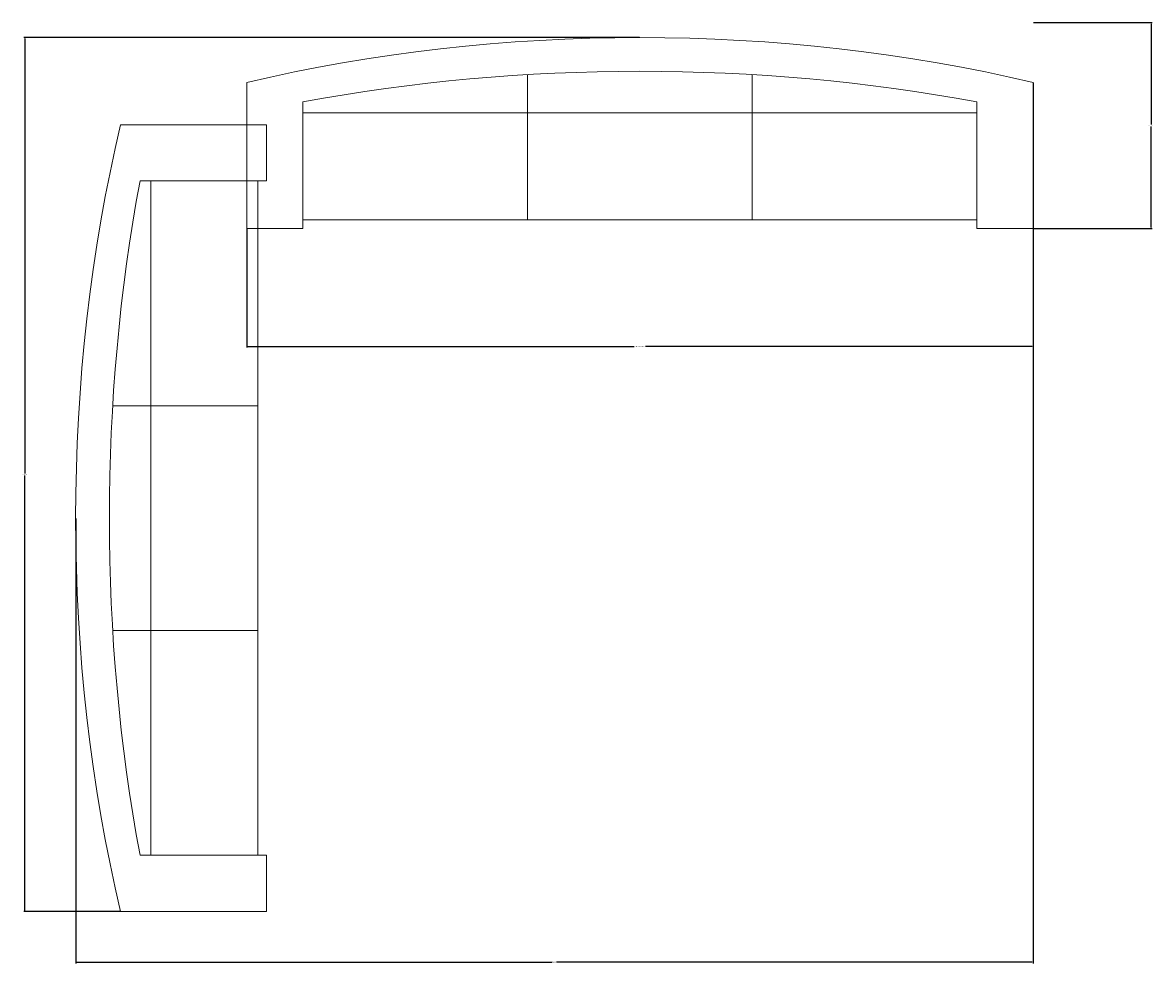
# Model space of a CAD drawing. Units: feet. Extents: x 2128 to 3163, y 1733 to 2266.
# Tile 1 of 3: x 2128 to 2322, y 1913 to 2074. Entities that reach past the tile are written whole.
import ezdxf

# ---------------------------------------------------------------- set-up
doc = ezdxf.new("R2010")
doc.units = ezdxf.units.FT
doc.layers.add('A-ANNO-DIMS', color=2, linetype='Continuous', lineweight=18)
doc.layers.add('A-FURN', color=8, linetype='Continuous', lineweight=18)
doc.styles.get("Standard").update_dxf_attribs({"font": 'arial.ttf'})
doc.dimstyles.get("Standard").update_dxf_attribs({"dimtxt": 0.18, "dimasz": 0.18, "dimexe": 0.18, "dimexo": 0.0625, "dimgap": 0.09, "dimtad": 0, "dimtih": 1, "dimtoh": 1, "dimdec": 4, "dimzin": 0, "dimdsep": 46, "dimtxsty": 'Standard', "dimcen": 0.09, "dimadec": 0, "dimazin": 0, "dimtfac": 1, "dimtdec": 4, "dimtofl": 0, "dimtmove": 0, "dimatfit": 3, "dimfxl": 1, "dimtolj": 1, "dimtzin": 0, "dimarcsym": 0})

# ---------------------------------------------------------------- blocks, each defined once
blk = doc.blocks.new('Sofa - Roundback 7 ft.')
for p, q in [((-12.00002, -32.4421), (-12.00003, -6.5971)), ((11.99997, -32.4421), (11.99998, -6.5971)), ((-36.000027, -34), (-36.000027, -11.4696)), ((35.99998, -34), (35.99998, -11.4696)), ((-35.999844, -13.3819), (35.9998, -13.3819)), ((-36.000027, -32.4421), (35.99998, -32.4421))]:
    blk.add_line(p, q)
for points in [[(-36.000027, -34), (-42.000027, -34), (-42.000027, -8)], [(41.99998, -8), (41.99998, -34), (35.99998, -34)]]:
    blk.add_lwpolyline(points)
for centre, radius, start, end in [((0, -114.25), 114.25, 68.43141, 111.5686), ((-0.00001, -127.1968), 121.1968, 72.72033, 107.2797)]:
    blk.add_arc(centre, radius, start, end)
blk = doc.blocks.new('*D11')
at = {"layer": 'A-ANNO-DIMS', "color": 0, "lineweight": -2, "transparency": 16777216}
for p, q in [((2166.47, 2038.29), (2166.47, 2018)), ((2301, 2038.29), (2301, 2018)), ((2166.65, 2018.18), (2232.76, 2018.18)), ((2300.82, 2018.18), (2234.71, 2018.18))]:
    blk.add_line(p, q, dxfattribs=at)
at = {"layer": 'A-ANNO-DIMS', "color": 0, "transparency": 16777216}
for points in [[(2166.65, 2018.21), (2166.65, 2018.15), (2166.47, 2018.18)], [(2300.82, 2018.21), (2300.82, 2018.15), (2301, 2018.18)]]:
    blk.add_solid(points, dxfattribs=at)
at = {"layer": 'Defpoints', "color": 0, "transparency": 16777216}
for p in [(2166.47, 2038.36), (2301, 2038.36), (2301, 2018.18)]:
    blk.add_point(p, dxfattribs=at)
at = {"layer": 'A-ANNO-DIMS', "color": 0, "transparency": 16777216, "insert": (2233.73, 2018.18), "char_height": 0.18, "attachment_point": 5}
blk.add_mtext('\\A1;SOFA 135 TYP.', dxfattribs=at)
blk = doc.blocks.new('*D12')
at = {"layer": 'A-ANNO-DIMS', "color": 0, "lineweight": -2, "transparency": 16777216}
for p, q in [((2301.06, 2073.56), (2321.36, 2073.56)), ((2321.18, 2073.38), (2321.18, 2056.14)), ((2321.18, 2038.54), (2321.18, 2055.78)), ((2301.06, 2038.36), (2321.36, 2038.36))]:
    blk.add_line(p, q, dxfattribs=at)
at = {"layer": 'A-ANNO-DIMS', "color": 0, "transparency": 16777216}
for points in [[(2321.15, 2073.38), (2321.21, 2073.38), (2321.18, 2073.56)], [(2321.15, 2038.54), (2321.21, 2038.54), (2321.18, 2038.36)]]:
    blk.add_solid(points, dxfattribs=at)
at = {"layer": 'Defpoints', "color": 0, "transparency": 16777216}
for p in [(2301, 2073.56), (2321.18, 2073.56), (2301, 2038.36)]:
    blk.add_point(p, dxfattribs=at)
at = {"layer": 'A-ANNO-DIMS', "color": 0, "transparency": 16777216, "insert": (2321.18, 2055.96), "char_height": 0.18, "attachment_point": 5}
blk.add_mtext('\\A1;35 TYP.', dxfattribs=at)
blk = doc.blocks.new('*D50')
at = {"layer": 'A-ANNO-DIMS', "color": 0, "lineweight": -2, "transparency": 16777216}
for p, q in [((2301, 2063.26), (2301, 1912.69)), ((2137.21, 1988.77), (2137.21, 1912.69)), ((2137.39, 1912.87), (2218.72, 1912.87)), ((2300.82, 1912.87), (2219.49, 1912.87))]:
    blk.add_line(p, q, dxfattribs=at)
at = {"layer": 'A-ANNO-DIMS', "color": 0, "transparency": 16777216}
for points in [[(2137.39, 1912.9), (2137.39, 1912.84), (2137.21, 1912.87)], [(2300.82, 1912.9), (2300.82, 1912.84), (2301, 1912.87)]]:
    blk.add_solid(points, dxfattribs=at)
at = {"layer": 'Defpoints', "color": 0, "transparency": 16777216}
for p in [(2301, 2063.32), (2137.21, 1988.83), (2301, 1912.87)]:
    blk.add_point(p, dxfattribs=at)
at = {"layer": 'A-ANNO-DIMS', "color": 0, "transparency": 16777216, "insert": (2219.1, 1912.87), "char_height": 0.18, "attachment_point": 5}
blk.add_mtext('\\A1;163.8', dxfattribs=at)
blk = doc.blocks.new('*D51')
at = {"layer": 'A-ANNO-DIMS', "color": 0, "lineweight": -2, "transparency": 16777216}
for p, q in [((2233.67, 2071), (2128.33, 2071)), ((2128.51, 2070.82), (2128.51, 1996.46)), ((2128.51, 1921.75), (2128.51, 1996.1)), ((2144.83, 1921.57), (2128.33, 1921.57))]:
    blk.add_line(p, q, dxfattribs=at)
at = {"layer": 'A-ANNO-DIMS', "color": 0, "transparency": 16777216}
for points in [[(2128.48, 2070.82), (2128.54, 2070.82), (2128.51, 2071)], [(2128.48, 1921.75), (2128.54, 1921.75), (2128.51, 1921.57)]]:
    blk.add_solid(points, dxfattribs=at)
at = {"layer": 'Defpoints', "color": 0, "transparency": 16777216}
for p in [(2128.51, 2071), (2233.73, 2071), (2144.89, 1921.57)]:
    blk.add_point(p, dxfattribs=at)
at = {"layer": 'A-ANNO-DIMS', "color": 0, "transparency": 16777216, "insert": (2128.51, 1996.28), "char_height": 0.18, "attachment_point": 5}
blk.add_mtext('\\A1;149.43', dxfattribs=at)

msp = doc.modelspace()

# ---------------------------------------------------------------- block references
at = {"layer": 'A-FURN', "xscale": 1.601553536944322, "yscale": 0.9600654288777931, "zscale": 1.601553536944322}
msp.add_blockref('Sofa - Roundback 7 ft.', (2233.732, 2070.9989), dxfattribs=at)
at = {"layer": 'A-FURN', "xscale": 1.601553536944322, "yscale": 0.9600654288777931, "zscale": 1.601553536944322, "rotation": 90}
msp.add_blockref('Sofa - Roundback 7 ft.', (2137.2083, 1988.8322), dxfattribs=at)

# ---------------------------------------------------------------- dimensions: what is measured, and where the dimension line sits
at = {"layer": 'A-ANNO-DIMS'}
dim = msp.add_linear_dim(base=(2321.1769, 2073.5591), p1=(2300.9973, 2038.3567), p2=(2300.9973, 2073.5591), angle=90, text='<> TYP.', dimstyle='Standard', override={"dimdec": 0, "dimlfac": 1, "dimrnd": 0, "dimzin": 0, "dimdsep": 46, "dimlunit": 2}, dxfattribs=at)
dim.commit()
dim.dimension.update_dxf_attribs({"geometry": '*D12', "text_midpoint": (2321.1769, 2055.9579)})
dim = msp.add_linear_dim(base=(2128.5083, 2070.9989), p1=(2144.8889, 1921.5669), p2=(2233.732, 2070.9989), angle=90, dimstyle='Standard', override={"dimdec": 2, "dimlfac": 1, "dimrnd": 0, "dimzin": 0, "dimdsep": 46, "dimlunit": 2}, dxfattribs=at)
dim.commit()
dim.dimension.update_dxf_attribs({"geometry": '*D51', "text_midpoint": (2128.5083, 1996.2829)})
dim = msp.add_linear_dim(base=(2300.9973, 1912.8669), p1=(2137.2083, 1988.8322), p2=(2300.9973, 2063.3184), dimstyle='Standard', override={"dimdec": 1, "dimlfac": 1, "dimrnd": 0, "dimzin": 0, "dimdsep": 46, "dimlunit": 2}, dxfattribs=at)
dim.commit()
dim.dimension.update_dxf_attribs({"geometry": '*D50', "text_midpoint": (2219.1028, 1912.8669)})
dim = msp.add_linear_dim(base=(2300.9973, 2018.1771), p1=(2166.4668, 2038.3567), p2=(2300.9973, 2038.3567), text='SOFA <> TYP.', dimstyle='Standard', override={"dimdec": 0, "dimlfac": 1, "dimrnd": 0, "dimzin": 0, "dimdsep": 46, "dimlunit": 2}, dxfattribs=at)
dim.commit()
dim.dimension.update_dxf_attribs({"geometry": '*D11', "text_midpoint": (2233.732, 2018.1771)})

doc.saveas('drawing.dxf')
